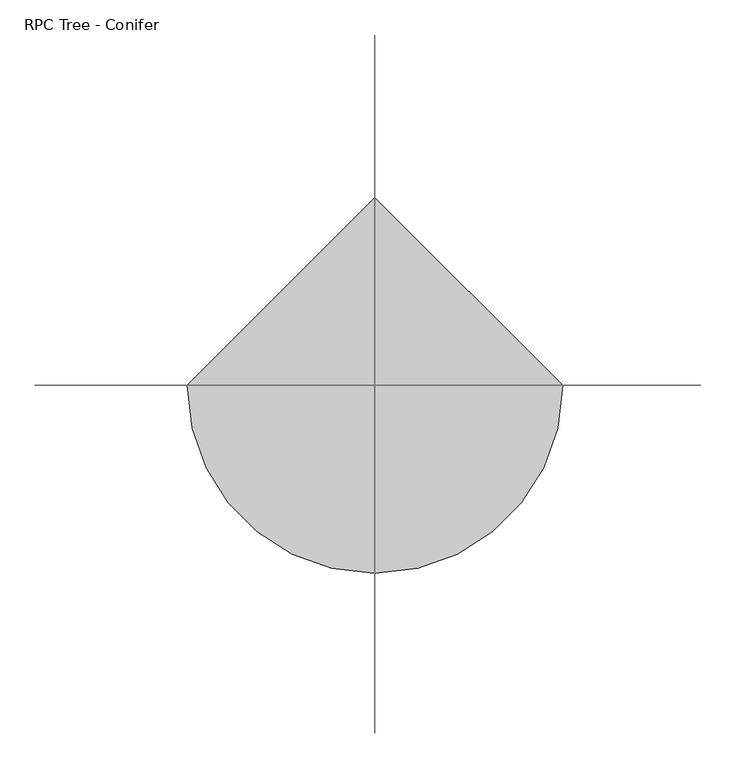
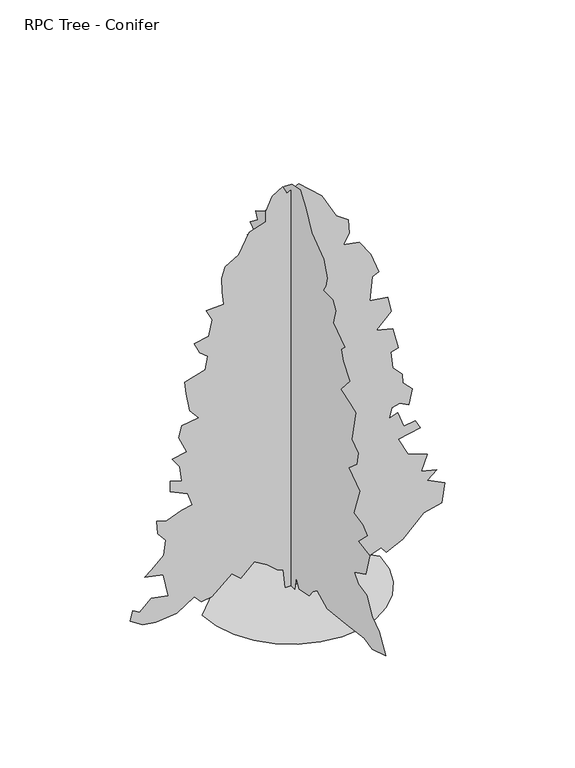
"""IFC4 building model written with IfcOpenShell, lengths in millimetres: geographic element geometry, RPC Tree - Conifer."""

from ifc_helpers import new_model, si_unit, origin, place, context, project, spatial, triangles, source, transform, mapped, element, save


def rpc_tree_conifer_97aab292(model_context):
    return source(origin(), model_context, "Body", "Tessellation", [
        triangles([(0.1966733, 49.3561489, 3.58e-05), (0.1966807, 76.1744156, 207.8417467), (0.196685, 109.6973104, 301.7045676), (0.1966884, 230.379379, 234.6600225), (0.1966932, 377.8792239, 174.3188474), (0.1966999, 545.4937022, 147.5005898), (0.1967076, 713.5737408, 154.6348927), (0.196705, 733.2223234, 40.2275228), (0.1967129, 853.9046373, 120.682323), (0.196716, 981.9569956, 35.9934516), (0.1967211, 1075.1551586, 67.0457895), (0.196729, 1256.1798649, 60.3411615), (0.1967353, 1343.3377716, 140.7959572), (0.1967491, 1531.0664291, 321.8186923), (0.1967456, 1417.0879211, 375.4547353), (0.1967421, 1316.5197865, 408.9791061), (0.1967377, 1222.8412022, 401.1533847), (0.19674, 1202.5413511, 509.5473135), (0.196744, 1229.359409, 603.4116059), (0.1967514, 1323.2237377, 710.6836555), (0.1967478, 1229.359409, 730.7978348), (0.1967531, 1303.1095585, 797.8441057), (0.196749, 1189.1335939, 831.3659695), (0.1967454, 1068.45128, 891.7084345), (0.1967463, 1006.4049946, 1015.8652456), (0.1967546, 1162.3155361, 1059.3228401), (0.1967594, 1229.359409, 1119.6627617), (0.1967561, 1142.2014296, 1139.7769409), (0.1967521, 994.7010578, 1226.9373184), (0.1967585, 1101.9731438, 1280.5734341), (0.1967642, 1110.6508118, 1457.1305351), (0.1967592, 987.9947084, 1475.0058975), (0.1967552, 880.7226225, 1501.8238827), (0.1967595, 896.547456, 1623.9847401), (0.1967665, 1027.1927519, 1660.8127247), (0.1967716, 1055.0409794, 1790.1206749), (0.1967662, 947.7689661, 1770.0064957), (0.1967671, 880.024264, 1900.4932983), (0.1967731, 954.4728447, 1991.2570896), (0.1967713, 860.6085159, 2071.7111904), (0.1967775, 954.4728447, 2138.7573887), (0.1967803, 981.2908298, 2192.3935043), (0.196776, 813.6763515, 2299.6680611), (0.1967771, 793.562245, 2366.7117886), (0.1967851, 927.6547869, 2433.7581322), (0.196785, 867.3123945, 2520.9283928), (0.1967808, 733.2223234, 2581.2558151), (0.1967877, 820.3802301, 2681.8267113), (0.1967861, 726.515974, 2768.9745895), (0.1967833, 605.8360946, 2856.1474663), (0.1967862, 599.1297452, 2963.42929), (0.1967921, 699.6979162, 3010.3589836), (0.1967904, 625.9502375, 3064.0001862), (0.1967871, 538.7898236, 3084.1091331), (0.1967946, 652.7682226, 3164.5460838), (0.196792, 532.085945, 3258.4301788), (0.1967955, 565.6078451, 3325.4691101), (0.1967916, 424.8113883, 3405.9304779), (0.1967901, 310.832953, 3526.610321), (0.1967913, 235.627587, 3681.4162788), (0.1967901, 96.2880544, 3848.4313751), (0.1967879, -10.9852091, 3935.5795441), (0.1967827, -145.0765916, 3962.4), (0.1967749, -238.9406479, 3841.7201569), (0.1967651, -332.804468, 3654.0013824), (0.1967522, -527.2369314, 3513.1875938), (0.1967452, -580.8729744, 3359.0007843), (0.1967436, -554.0549529, 3265.1166893), (0.1967433, -520.5330528, 3204.7889763), (0.1967367, -668.0334246, 3204.7889763), (0.1967322, -714.9655163, 3124.3276085), (0.1967298, -674.7373032, 2983.5385277), (0.1967176, -862.465888, 2856.1474663), (0.1967187, -802.1234957, 2802.5065544), (0.1967143, -835.6479029, 2701.9356583), (0.1967057, -942.9199162, 2574.5445969), (0.1967072, -795.4196171, 2406.9400017), (0.1966989, -950.7208935, 2358.4253757), (0.1966939, -1036.7842449, 2319.782095), (0.1966878, -976.4418526, 2024.779026), (0.1966811, -1077.0125307, 1951.0287312), (0.1966784, -1056.8983515, 1830.3464172), (0.1966807, -929.5096882, 1716.3705254), (0.1966693, -1103.8305159, 1595.6882114), (0.1966656, -1003.2623085, 1320.7991764), (0.1966582, -1150.7626802, 1293.9811913), (0.1966531, -1224.5129025, 1233.6412697), (0.1966553, -1077.0125307, 1086.1408979), (0.1966461, -1264.7386448, 1059.3228401), (0.1966425, -1197.6948446, 838.0699207), (0.196648, -1016.6701384, 750.9119413), (0.1966429, -1077.0125307, 670.4579132), (0.1966358, -1217.8064804, 643.6398554), (0.1966273, -1304.9668579, 489.4331706), (0.1966198, -1418.9453659, 408.9791061), (0.1966101, -1519.5135006, 234.6600225), (0.1966177, -1304.9668579, 167.614224), (0.1966245, -1173.3830292, 197.6893322), (0.1966363, -887.0773218, 162.532194), (0.1966489, -580.8729744, 127.3867012), (0.1966585, -419.962411, 207.8417467), (0.1966599, -352.9185745, 154.204977), (0.1966604, -292.5761822, 80.4548002), (0.1966666, -131.6673356, 46.9321508), (0.1966712, -85.0868485, 132.0635687), (0.1966685, -57.9171634, 3.26e-05), (-50.7214044, 1.3e-06, 3.59e-05), (-70.8350431, -2.06e-05, 181.023489), (-124.4715721, -1.99e-05, 201.1371233), (-218.3356374, -2.07e-05, 281.5929136), (-339.0169521, -2.04e-05, 355.3430632), (-466.4056518, 3.2e-06, 234.6600225), (-546.8596799, 2.3e-06, 308.4109351), (-734.5883011, 1.51e-05, 147.5005898), (-828.8563116, 1.84e-05, 135.7027906), (-895.49643, 1.72e-05, 207.8417467), (-1056.4070297, 2.68e-05, 100.5686797), (-1250.8394932, 4.79e-05, 80.4550455), (-1371.5218071, 5.06e-05, 100.5686797), (-1485.5003151, 5.07e-05, 174.3188474), (-1465.3861359, 4.59e-05, 268.1826675), (-1398.3397923, 4.57e-05, 227.9553809), (-1291.0653809, 2.36e-05, 328.525078), (-1136.8610579, 2.02e-05, 301.7045676), (-1182.3370611, 1.16e-05, 523.1482275), (-1351.4077732, 1.52e-05, 556.4794415), (-1291.0653809, 1.13e-05, 603.4116059), (-1177.0893436, 3.1e-06, 710.6836555), (-1156.9752371, -3.8e-06, 851.4801487), (-1230.7254593, -5.5e-06, 938.6405262), (-1244.1356873, -1.08e-05, 1066.0267914), (-1150.2713585, -1.24e-05, 1039.2087336), (-1009.4748653, -3.34e-05, 1092.8447765), (-915.6106092, -3.71e-05, 1112.9588831), (-955.8388224, -4.13e-05, 1233.6412697), (-1116.8906199, -3.98e-05, 1309.0705318), (-1116.7469513, -4.46e-05, 1414.6635052), (-1009.4748653, -4.63e-05, 1381.1415688), (-1027.5656942, -5.21e-05, 1523.6492947), (-1096.6353155, -5.44e-05, 1622.5061966), (-962.542701, -5.96e-05, 1649.3241817), (-1036.2929232, -6.46e-05, 1810.2323833), (-1009.4748653, -7.02e-05, 1917.5069401), (-855.2706877, -9.04e-05, 1944.3249252), (-935.7247158, -9.22e-05, 2038.189254), (-969.2465796, -9.93e-05, 2219.2114895), (-982.6568802, -0.000104, 2333.1898521), (-794.9282227, -0.0001123, 2393.5297737), (-768.1102375, -0.0001185, 2514.2171745), (-841.860387, -0.000119, 2574.5445969), (-895.49643, -0.0001222, 2681.8267113), (-759.157659, -0.0001417, 2704.7837402), (-727.8819517, -0.0001494, 2856.1474663), (-781.5179947, -0.0001526, 2963.42929), (-620.6098658, -0.0001577, 2970.1160912), (-634.0176956, -0.0001629, 3097.5071526), (-640.724045, -0.0001687, 3231.6097229), (-607.1996015, -0.0001742, 3332.1803284), (-482.926373, -0.0001957, 3408.5803162), (-385.9491165, -0.0002069, 3593.6492523), (-231.7446482, -0.0002136, 3640.5789459), (-231.7446482, -0.0002181, 3741.1495514), (-171.4034912, -0.0002256, 3868.5406128), (-77.5396711, -0.0002311, 3928.8683258), (-37.3121507, -0.000229, 3855.1178856), (69.9609141, -0.000249, 3908.7590881), (284.5062896, -0.0002467, 3714.3290955), (418.5988678, -0.0002255, 3472.9694092), (532.5773031, -0.0002397, 3392.5077507), (539.2812181, -0.0002195, 3258.4301788), (485.6451751, -0.0002137, 3164.5460838), (633.1454378, -0.0002169, 3137.7503357), (740.4175238, -0.0002132, 2983.5385277), (814.167746, -0.0002067, 2789.108535), (753.1764833, -0.0002035, 2757.3845993), (727.0097666, -0.0001927, 2534.3264122), (894.6217741, -0.0001965, 2507.5056656), (928.1461813, -0.0001909, 2360.0079826), (787.3496881, -0.0001807, 2225.9177662), (941.5539385, -0.0001835, 2185.6895531), (995.1924522, -0.0001614, 1977.8468616), (921.4397593, -0.0001587, 1964.4391045), (941.5539385, -0.0001521, 1803.5284321), (1030.220038, -0.0001504, 1706.6750416), (1035.4181946, -0.0001468, 1622.5061966), (1122.5786448, -0.0001455, 1535.3458191), (1089.0542376, -0.0001379, 1387.84552), (1008.6002094, -0.0001376, 1434.7775391), (934.8500599, -0.0001345, 1414.6635052), (908.0320021, -0.0001295, 1320.7991764), (988.4861029, -0.0001331, 1347.6171616), (1042.1220732, -0.0001278, 1193.4129839), (1149.3966299, -0.0001319, 1213.5270905), (1196.3287943, -0.0001294, 1126.366713), (995.1924522, -0.0001216, 1086.1408979), (1082.350359, -0.000102, 911.8200703), (1263.3750652, -0.0001188, 844.7762701), (1205.4472784, -9.61e-05, 697.2783691), (1350.532972, -9.89e-05, 663.7515638), (1263.3750652, -9.3e-05, 590.001378), (1424.2832668, -9.42e-05, 509.5473135), (1397.4651363, -8.5e-05, 321.8186923), (1229.850658, -7.82e-05, 281.5929136), (1036.3395046, -6.4e-05, 93.3593451), (881.2140169, -4.18e-05, 20.1136387), (834.2818525, -4.31e-05, 80.4548002), (658.291868, -3.51e-05, 20.7551739), (472.2349108, -2.93e-05, 13.4091084), (398.4847612, -3.01e-05, 80.4548002), (230.8705009, -2.78e-05, 140.7959572), (72.6778858, -2.16e-05, 108.3902136), (56.5516581, -1.63e-05, 3.27e-05), (-820.443671, -4.5e-06, 5.88e-05), (-798.7470303, -188.0361787, 5.26e-05), (-736.9608307, -360.7170811, 4.56e-05), (-640.0281572, -513.0961158, 3.82e-05), (-512.8994345, -640.2248022, 3.06e-05), (-360.5203998, -737.1574757, 2.32e-05), (-187.8395156, -798.9436752, 1.62e-05), (0.1967069, -820.640316, 9.9e-06), (188.2328419, -798.9436752, 5e-06), (360.9137624, -737.1574757, 1.7e-06), (513.2927971, -640.2248022, 0.0), (640.4214472, -513.0961158, 0.0), (737.3541206, -360.7170811, 1.7e-06), (799.1403202, -188.0361787, 5e-06), (820.836961, 7.6e-05, 9.9e-06), (0.1965635, 820.640316, 5.88e-05)], [[26, 27, 28], [21, 22, 23], [19, 20, 21], [51, 52, 53], [7, 8, 9], [35, 36, 37], [13, 14, 15], [34, 35, 37], [54, 55, 56], [72, 73, 74], [95, 96, 97], [88, 89, 90], [44, 45, 46], [86, 87, 88], [85, 86, 88], [51, 53, 54], [44, 46, 47], [88, 90, 91], [13, 15, 16], [13, 16, 17], [38, 39, 40], [25, 26, 28], [25, 28, 29], [47, 48, 49], [56, 57, 58], [30, 31, 32], [29, 30, 32], [41, 42, 43], [40, 41, 43], [106, 1, 2], [105, 106, 2], [75, 76, 77], [94, 95, 97], [94, 97, 98], [78, 79, 80], [83, 84, 85], [29, 32, 33], [103, 104, 105], [12, 13, 17], [11, 12, 17], [77, 78, 80], [102, 103, 105], [62, 63, 64], [80, 81, 82], [80, 82, 83], [61, 62, 64], [61, 64, 65], [60, 61, 65], [59, 60, 65], [69, 70, 71], [69, 71, 72], [94, 98, 99], [93, 94, 99], [92, 93, 99], [92, 99, 100], [91, 92, 100], [91, 100, 101], [47, 49, 50], [9, 10, 11], [9, 11, 17], [9, 17, 18], [7, 9, 18], [59, 65, 66], [59, 66, 67], [59, 67, 68], [59, 68, 69], [58, 59, 69], [56, 58, 69], [54, 56, 69], [54, 69, 72], [51, 54, 72], [50, 51, 72], [50, 72, 74], [50, 74, 75], [50, 75, 77], [47, 50, 77], [44, 47, 77], [43, 44, 77], [40, 43, 77], [40, 77, 80], [40, 80, 83], [38, 40, 83], [38, 83, 85], [37, 38, 85], [34, 37, 85], [33, 34, 85], [29, 33, 85], [25, 29, 85], [25, 85, 88], [25, 88, 91], [25, 91, 101], [25, 101, 102], [24, 25, 102], [23, 24, 102], [21, 23, 102], [105, 2, 3], [102, 105, 3], [21, 102, 3], [21, 3, 4], [21, 4, 5], [21, 5, 6], [21, 6, 7], [21, 7, 18], [19, 21, 18], [125, 126, 127], [198, 199, 200], [153, 154, 155], [139, 140, 141], [130, 131, 132], [120, 121, 122], [119, 120, 122], [186, 187, 188], [136, 137, 138], [135, 136, 138], [150, 151, 152], [193, 194, 195], [192, 193, 195], [125, 127, 128], [180, 181, 182], [163, 164, 165], [185, 186, 188], [196, 197, 198], [190, 191, 192], [111, 112, 113], [212, 107, 108], [211, 212, 108], [173, 174, 175], [149, 150, 152], [179, 180, 182], [129, 130, 132], [146, 147, 148], [204, 205, 206], [200, 201, 202], [200, 202, 203], [162, 163, 165], [190, 192, 195], [165, 166, 167], [118, 119, 122], [118, 122, 123], [118, 123, 124], [117, 118, 124], [116, 117, 124], [176, 177, 178], [176, 178, 179], [129, 132, 133], [185, 188, 189], [142, 143, 144], [141, 142, 144], [161, 162, 165], [161, 165, 167], [161, 167, 168], [116, 124, 125], [145, 146, 148], [144, 145, 148], [114, 115, 116], [113, 114, 116], [113, 116, 125], [113, 125, 128], [113, 128, 129], [113, 129, 133], [113, 133, 134], [111, 113, 134], [168, 169, 170], [168, 170, 171], [161, 168, 171], [160, 161, 171], [159, 160, 171], [158, 159, 171], [157, 158, 171], [156, 157, 171], [155, 156, 171], [171, 172, 173], [171, 173, 175], [155, 171, 175], [155, 175, 176], [153, 155, 176], [152, 153, 176], [149, 152, 176], [149, 176, 179], [148, 149, 179], [144, 148, 179], [144, 179, 182], [144, 182, 183], [141, 144, 183], [139, 141, 183], [138, 139, 183], [135, 138, 183], [134, 135, 183], [111, 134, 183], [110, 111, 183], [110, 183, 184], [110, 184, 185], [110, 185, 189], [110, 189, 190], [110, 190, 195], [109, 110, 195], [108, 109, 195], [211, 108, 195], [210, 211, 195], [210, 195, 196], [209, 210, 196], [209, 196, 198], [208, 209, 198], [207, 208, 198], [206, 207, 198], [204, 206, 198], [203, 204, 198], [200, 203, 198], [227, 228, 213], [226, 227, 213], [226, 213, 214], [225, 226, 214], [225, 214, 215], [225, 215, 216], [224, 225, 216], [223, 224, 216], [223, 216, 217], [223, 217, 218], [223, 218, 219], [223, 219, 220], [223, 220, 221], [223, 221, 222]], closed=False),
    ])


if __name__ == "__main__":
    model = new_model("IFC4")
    model_context = context("Model", 3, world=origin())
    ifc_project = project(units=[si_unit("LENGTHUNIT", "METRE", prefix="MILLI")], contexts=[model_context])
    site = spatial("IfcSite", under=ifc_project)
    building = spatial("IfcBuilding", under=site)
    placement = place(None, origin())
    rpc_tree_conifer_shape = rpc_tree_conifer_97aab292(model_context)
    element("IfcGeographicElement", 1, ObjectType="RPC Tree - Conifer", at=placement, inside=building, context=model_context, shape_type="MappedRepresentation", body=[
        mapped(rpc_tree_conifer_shape, transform((0.0, 0.0, 0.0), x_axis=(1.0, 0.0, 0.0), y_axis=(0.0, 1.0, 0.0), z_axis=(0.0, 0.0, 1.0))),
    ])
    save(model, "model.ifc")

# Revit data of these elements
# Type "RPC Tree - Conifer"
#   built-in parameter 1005198 = "{2, 15},{39, RPC-16-G0M4-N9PX-U6TN-C000-ST1L-LVER-AU},{1, 0},{1, 0},{2, 13},{1, 8},{5, Color},{1, 0},{1, 0},{3, 0.8},{3, 0.8},{3, 0.8},{1, 8},{7, BBoxMin},{1, 0},{1, 0},{1, 0},{1, 0},{1, 0},{1, 8},{7, BBoxMax},{1, 0},{1, 0},{1, 0},{1, 0},{1, 0},{2, 11},{9, RPCTypeId},{1, 0},{1, 0},{39, RPC-16-G0M4-N9PX-U6TN-C000-ST1L-LVER-AU},{1, 6},{14, RPCPlantHeight},{1, 0},{1, 0},{2, 13},{2, 11},{7, keyword},{1, 0},{1, 0},{34, :RPCs:Trees [General]:Geometry:RPC},{2, 11},{8, category},{1, 0},{1, 0},{15, Trees [General]},{2, 11},{12, LocalizedUID},{1, 0},{1, 0},{15, Colorado Spruce},{2, 14},{6, Height},{1, 0},{1, 0},{2, 13},{1, 2},{16, Cast Reflections},{1, 0},{1, 0},{1, 0},{1, 2},{12, Cast Shadows},{1, 0},{1, 0},{1, 1},{1, 2},{9, Lock View},{1, 0},{1, 0},{1, 0},{1, 4},{5, ViewC},{1, 0},{1, 0},{1, 0},{21, assetlibrary_base.fbx},{1, 5},"
#   built-in parameter 1005195 = "RPC-16-G0M4-N9PX-U6TN-C000-ST1L-LVER-AU"
#   Assembly Code = "G2050500"
#   Height = 13' - 0"
#   Description = (empty or 0)
#   Default Elevation = 0
